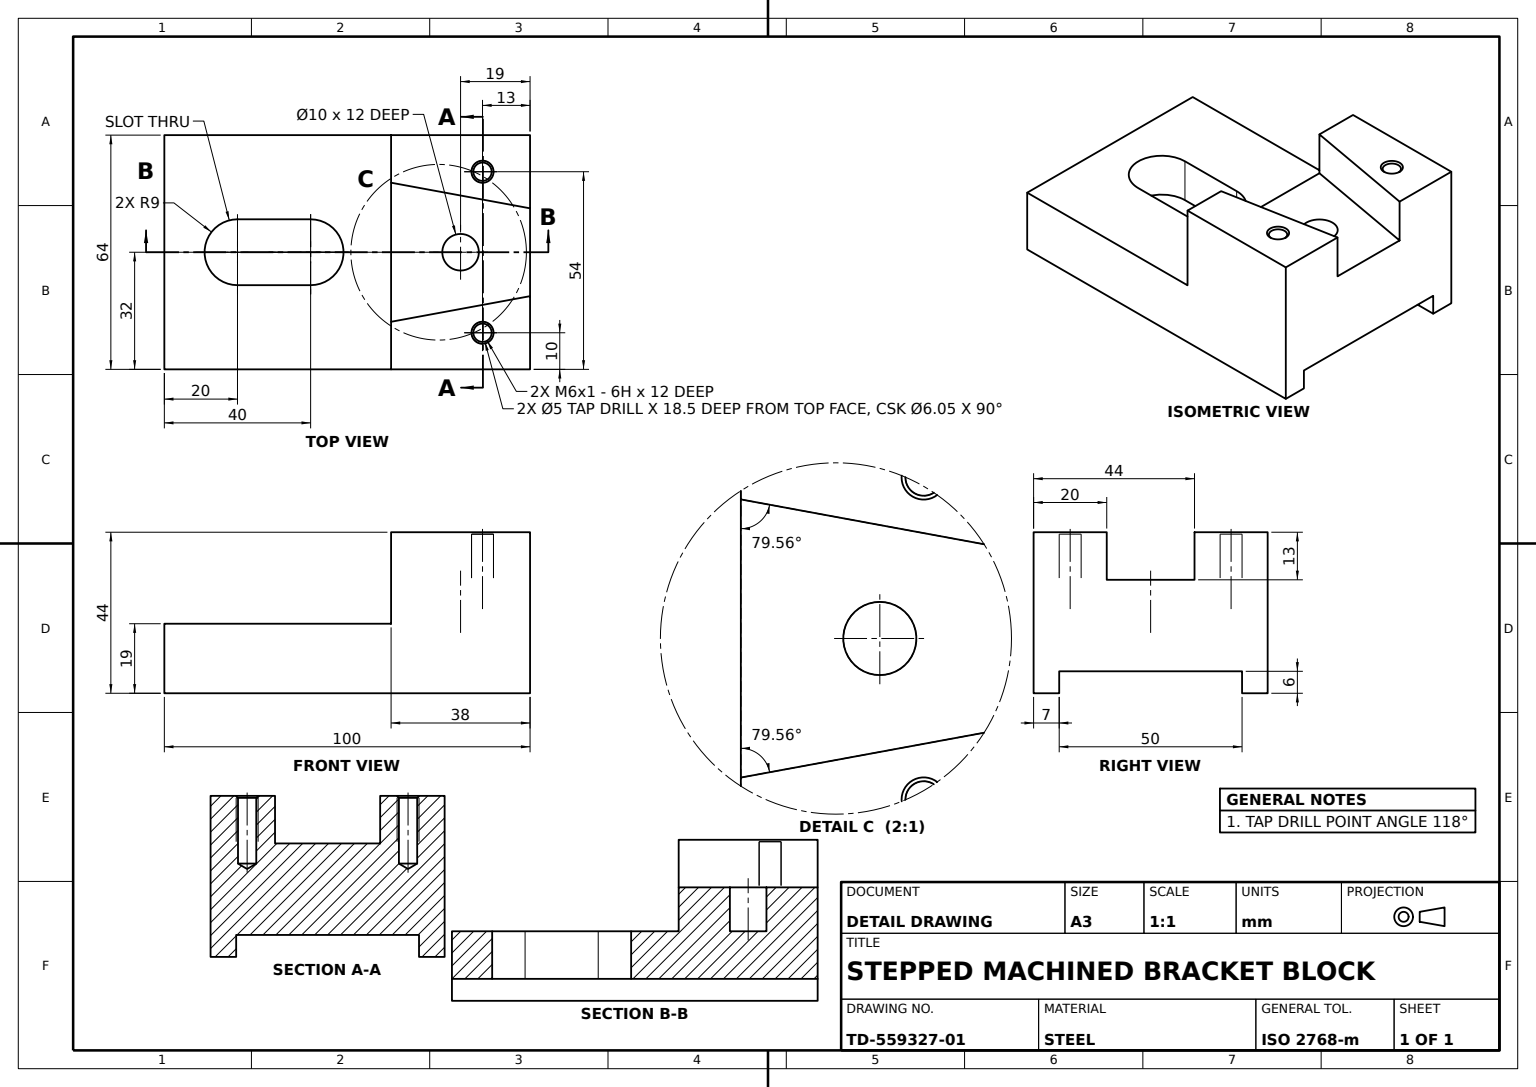
from build123d import *

# Parameters (mm, degrees)
BASE_PLATE_DEPTH                      = 100
V_BLOCK_UPRIGHTS_DEPTH                = 25
M6_TAPPED_HOLES_2X_D                  = 5
M6_TAPPED_HOLES_2X_DEPTH              = 18.497848452
M6_TAPPED_HOLES_2X_CSINK_D            = 6.05
M6_TAPPED_HOLES_2X_CSINK_ANGLE        = 90
M6_TAPPED_HOLES_2X_TIP                = 1.502151548
CENTRE_STEP_BLOCK_PROFILE_R           = 5
CENTRE_STEP_BLOCK_DEPTH               = 12
ADJUSTMENT_SLOT_AND_CENTRE_HOLE_DEPTH = 108.930533215


with BuildPart() as part:
    # Base Plate Profile → Base Plate (new body)
    with BuildSketch(Plane.XY):
        Polygon((25, 0), (-25, 0), (-25, -6), (-32, -6), (-32, 13), (32, 13), (32, -6), (25, -6), align=None)
    extrude(amount=-BASE_PLATE_DEPTH)

    # V-Block Uprights Profile → V-Block Uprights (add)
    with BuildSketch(Plane(origin=(0, 13, 0), x_dir=(1, 0, 0), z_dir=(0, 1, 0))):
        Polygon((32, 100), (32, 62), (19, 62), (12, 100), align=None)
        Polygon((-12, 100), (-32, 100), (-32, 62), (-19, 62), align=None)
    extrude(amount=V_BLOCK_UPRIGHTS_DEPTH)

    # M6 Tapped Holes 2x
    with Locations(Plane(origin=(0, 38, 0), x_dir=(1, 0, 0), z_dir=(0, 1, 0))):
        with Locations((22, 87), (-22, 87)):
            CounterSinkHole(M6_TAPPED_HOLES_2X_D / 2, M6_TAPPED_HOLES_2X_CSINK_D / 2, depth=M6_TAPPED_HOLES_2X_DEPTH, counter_sink_angle=M6_TAPPED_HOLES_2X_CSINK_ANGLE)
            with Locations((0, 0, -(M6_TAPPED_HOLES_2X_DEPTH + M6_TAPPED_HOLES_2X_TIP / 2))):  # 118° drill point
                Cone(0, M6_TAPPED_HOLES_2X_D / 2, M6_TAPPED_HOLES_2X_TIP, mode=Mode.SUBTRACT)

    # Centre Step Block Profile → Centre Step Block (add)
    with BuildSketch(Plane(origin=(0, 13, 0), x_dir=(1, 0, 0), z_dir=(0, 1, 0))):
        Polygon((-12, 100), (12, 100), (19, 62), (-19, 62), align=None)
        with Locations(Location((0, 81, 0), (0, 0, 180))):
            Circle(CENTRE_STEP_BLOCK_PROFILE_R, mode=Mode.SUBTRACT)
    extrude(amount=CENTRE_STEP_BLOCK_DEPTH)

    # Adjustment Slot and Centre Hole Profile → Adjustment Slot and Centre Hole (cut, through all)
    with BuildSketch(Plane(origin=(0, 13, 0), x_dir=(1, 0, 0), z_dir=(0, 1, 0))):
        with BuildLine():
            Line((-9, 20), (-9, 40))
            ThreePointArc((-9, 40), (0, 49), (9, 40))
            Line((9, 40), (9, 20))
            ThreePointArc((9, 20), (0, 11), (-9, 20))
        make_face()
    extrude(amount=-ADJUSTMENT_SLOT_AND_CENTRE_HOLE_DEPTH, mode=Mode.SUBTRACT)


solid = part.part
